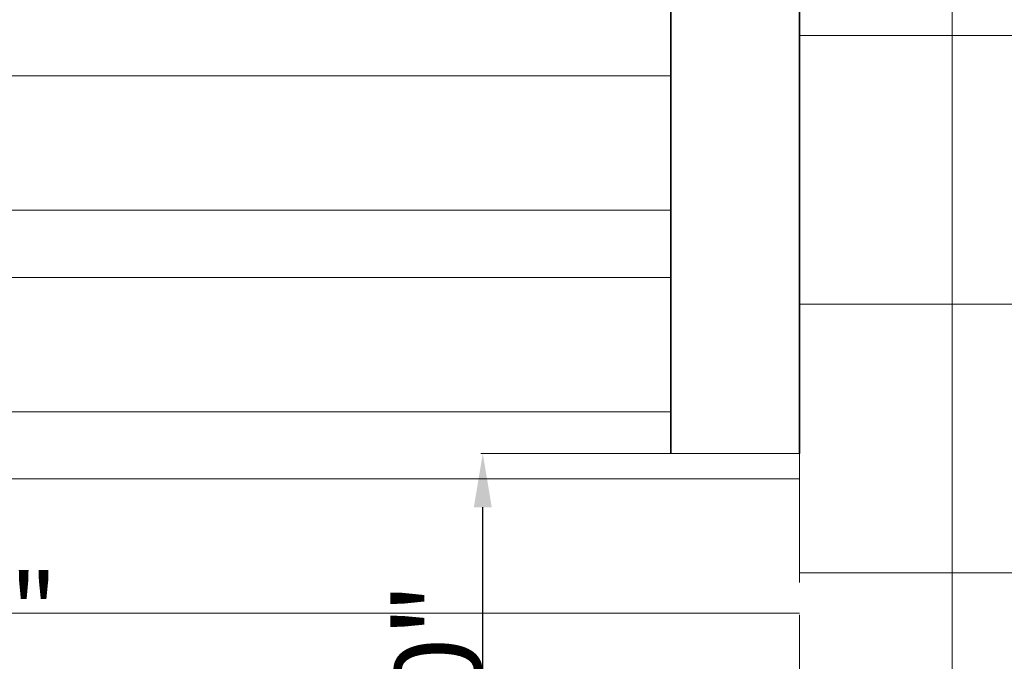
# Model space of a CAD drawing. Units: inches. Extents: x 351 to 1738, y -265 to 286.
# Tile 19 of 38: x 1176 to 1268, y -122 to -63. Entities that reach past the tile are written whole.
import ezdxf

# ---------------------------------------------------------------- set-up
doc = ezdxf.new("R2010")
doc.units = ezdxf.units.IN
doc.header["$MEASUREMENT"] = 0
doc.linetypes.add('ACAD_ISO02W100', pattern=[15, 12, -3])
for name, color, linetype, lineweight in [('A-ANNO-DIMS', 2, 'Continuous', 18), ('A-AREA-IDEN', 7, 'Continuous', 18), ('A-DOOR', 3, 'Continuous', 18), ('A-DOOR-OVHD', 3, 'ACAD_ISO02W100', 13), ('A-FLOR-PATT', 9, 'Continuous', 9), ('A-WALL', 7, 'Continuous', 35)]:
    doc.layers.add(name, color=color, linetype=linetype, lineweight=lineweight)
doc.styles.add('Annotative', font='arial.ttf')
doc.styles.get("Standard").update_dxf_attribs({"font": 'arial.ttf'})
doc.dimstyles.get("Standard").update_dxf_attribs({"dimtxt": 8, "dimasz": 5, "dimexe": 0.18, "dimexo": 0.0625, "dimgap": 0.09, "dimtad": 1, "dimtoh": 1, "dimzin": 0, "dimdsep": 46, "dimlunit": 4, "dimtxsty": 'Standard', "dimcen": 0, "dimclre": 256, "dimadec": 0, "dimazin": 0, "dimtfac": 1, "dimtofl": 0, "dimtmove": 0, "dimatfit": 3, "dimfxl": 1, "dimtolj": 1, "dimtzin": 0, "dimlwe": -1, "dimarcsym": 0})

# ---------------------------------------------------------------- blocks, each defined once
blk = doc.blocks.new('*D65')
at = {"layer": 'A-ANNO-DIMS', "transparency": 16777216}
for p, q in [((1248.45, -102.915), (1218.882, -102.915)), ((1248.45, -150.915), (1218.882, -150.915))]:
    blk.add_line(p, q, dxfattribs=at)
at = {"layer": 'A-ANNO-DIMS', "color": 0, "lineweight": -2, "transparency": 16777216}
blk.add_line((1219.062, -145.915), (1219.062, -107.915), dxfattribs=at)
at = {"layer": 'A-ANNO-DIMS', "color": 0, "transparency": 16777216}
for points in [[(1218.229, -107.915), (1219.896, -107.915), (1219.062, -102.915)], [(1218.229, -145.915), (1219.896, -145.915), (1219.062, -150.915)]]:
    blk.add_solid(points, dxfattribs=at)
at = {"layer": 'Defpoints', "color": 0, "transparency": 16777216}
for p in [(1219.062, -102.915), (1248.512, -102.915), (1248.512, -150.915)]:
    blk.add_point(p, dxfattribs=at)
at = {"layer": 'A-ANNO-DIMS', "color": 0, "transparency": 16777216, "insert": (1214.888, -126.915), "char_height": 8, "attachment_point": 5, "rotation": 90}
blk.add_mtext('\\A1;4\'-0"', dxfattribs=at)

msp = doc.modelspace()

# ---------------------------------------------------------------- hatches: boundary and pattern name
at = {"layer": 'A-FLOR-PATT', "transparency": 33554559}
h = msp.add_hatch(dxfattribs=at)
h.set_pattern_fill('ANSI37', color=256, scale=200, angle=135)
h.set_pattern_definition([(180, (1112.704, -164.037), (-2e-15, -25), []), (270, (1112.704, -164.037), (25, -5e-15), [])])
h.paths.add_polyline_path([(1380.064, 73.463), (1380.132, 148.463), (1338.064, 148.463), (1290.704, 148.463), (1290.704, 88.463), (1248.704, 88.463), (1248.704, -2.009), (1244.704, -2.009), (1244.704, 142.457), (1160.704, 142.457), (1160.704, 158.963), (1160.704, 170.137), (1160.704, 206.137), (1160.704, 228.963), (1112.704, 228.963), (1112.704, 209.963), (1112.704, 168.963), (1124.704, 168.963), (1124.704, 162.963), (1112.704, 162.963), (1112.704, 64.463), (1112.704, 60.463), (1112.704, 0.463), (1112.704, -48.026), (1146.804, -47.981), (1146.804, -35.691), (1207.804, -35.691), (1207.804, -47.902), (1236.542, -47.864), (1236.544, -50.009), (1248.5, -50.009), (1248.506, -102.915), (1248.512, -150.915), (1248.514, -164.037), (1248.549, -164.037), (1273.017, -164.037), (1273.017, -128.799), (1355.24, -128.799), (1355.24, -164.037), (1384.204, -164.037), (1384.204, -57.037), (1380.064, -57.037), (1380.064, -48.037), (1392.064, -48.037), (1392.064, -53.037), (1406.549, -53.037), (1406.549, -57.037), (1401.204, -57.037), (1401.204, -147.037), (1468.204, -147.037), (1468.204, -138.5), (1472.204, -138.5), (1472.204, -102.5), (1468.204, -102.5), (1468.204, -57.037), (1442.549, -57.037), (1442.549, -53.037), (1463.049, -53.037), (1463.049, -40.747), (1524.049, -40.747), (1524.049, -48.037), (1536.064, -48.037), (1536.064, -53.037), (1557.704, -53.037), (1557.704, 204.963), (1384.204, 204.963), (1384.204, 73.463), (1392.064, 73.463), (1392.064, 64.463), (1384.204, 64.463), (1384.204, -3.5), (1380.204, -3.537), (1380.204, 64.463), (1380.064, 64.463)])
h.paths.add_polyline_path([(1510.714, 86.458, -0.103984), (1511.661, 85.595, 0.470438), (1510.158, 87.614, 0.0961)], flags=16)
h.paths.add_polyline_path([(1510.443, 100.266, 0.009798), (1504.693, 100.48, 0.02879), (1504.6, 99.767, -0.165331), (1505.519, 96.135, -0.143601)], flags=16)
h.paths.add_polyline_path([(1487.201, 85.595, -0.103984), (1488.148, 86.458, 0.0961), (1488.704, 87.614, 0.470438)], flags=0)
h.paths.add_polyline_path([(1495.052, 100.43), (1494.178, 100.43, -0.026463), (1494.262, 99.774, -0.144219)], flags=16)
h.paths.add_polyline_path([(1444.485, 86.458, -0.103984), (1445.433, 85.595, 0.470438), (1443.93, 87.614, 0.0961)], flags=16)
h.paths.add_polyline_path([(1420.972, 85.595, -0.103984), (1421.92, 86.458, 0.0961), (1422.475, 87.614, 0.470438)], flags=16)
h.paths.add_polyline_path([(1428.632, 100.335, 0.001054), (1427.971, 100.309, -0.021524), (1428.033, 99.774, -0.114301)], flags=16)
h.paths.add_polyline_path([(1419.906, 143.708, 0.024979), (1420.222, 157.526), (1421.573, 159.101), (1421.573, 175.369), (1391.393, 175.369), (1391.393, 200.519), (1542.294, 200.519), (1542.294, 175.369), (1512.028, 175.369, 0.019865), (1511.521, 153.838, 0.025134), (1512.758, 118.323, 0.020553), (1512.942, 115.253), (1419.834, 115.253, -0.000414), (1419.843, 124.798), (1413.059, 124.798), (1413.059, 84.437, -0.061853), (1415.831, 80.45, -0.093077), (1420.972, 85.595, -0.267537), (1422.371, 84.732, 0.08511), (1424.052, 84.616, -0.885393), (1424.033, 84.851, -1.125815), (1424.073, 84.366, -0.087987), (1422.371, 84.732, -0.267537), (1422.326, 83.089, -0.370542), (1420.972, 85.595, 0.093077), (1415.831, 80.45, -0.087414), (1417.914, 73.937), (1418.941, 73.937, 0.02725), (1418.913, 76.906, -0.115703), (1421.051, 73.937), (1445.354, 73.937, -0.115703), (1447.492, 76.906, 0.02725), (1447.464, 73.937), (1448.491, 73.937, -0.087414), (1450.574, 80.45, 0.093077), (1445.433, 85.595, -0.370542), (1444.079, 83.089, -0.267537), (1444.034, 84.732, -0.087987), (1442.332, 84.366, -1.125815), (1442.372, 84.851, -2.032736), (1442.364, 84.368, 0.086378), (1444.034, 84.732, -0.267537), (1445.433, 85.595, -0.093077), (1450.574, 80.45, -0.257732), (1466.483, 90.927, -0.47867), (1468.832, 91.907, -0.47867), (1471.18, 90.927, -0.26264), (1483.053, 81.78, -0.071866), (1487.201, 85.595, -0.267537), (1488.6, 84.732, 0.08511), (1490.28, 84.616, -0.885393), (1490.262, 84.851, -1.125815), (1490.301, 84.366, -0.087987), (1488.6, 84.732, -0.267537), (1488.554, 83.089, -0.370542), (1487.201, 85.595, 0.071866), (1483.053, 81.78, -0.132065), (1484.143, 73.937), (1485.169, 73.937, 0.02725), (1485.142, 76.906, -0.115703), (1487.28, 73.937), (1511.582, 73.937, -0.115703), (1513.72, 76.906, 0.02725), (1513.693, 73.937), (1514.719, 73.937, -0.087414), (1516.802, 80.45, 0.093077), (1511.661, 85.595, -0.370542), (1510.308, 83.089, -0.267537), (1510.262, 84.732, -0.087987), (1508.561, 84.366, -1.125815), (1508.601, 84.851, -2.032736), (1508.592, 84.368, 0.086378), (1510.262, 84.732, -0.267537), (1511.661, 85.595, -0.093077), (1516.802, 80.45, -0.061853), (1519.575, 84.437), (1519.575, 73.937), (1413.059, 73.937), (1413.059, 124.798), (1419.843, 124.798, -0.000821)], flags=16)
h.paths.add_polyline_path([(1220.149, 54.133, -0.103984), (1220.869, 53.476, 0.470438), (1219.727, 55.011, 0.0961)], flags=16)
h.paths.add_polyline_path([(1219.944, 64.626, 0.009798), (1215.574, 64.789, 0.02879), (1215.503, 64.247, -0.165331), (1216.201, 61.487, -0.143601)], flags=16)
h.paths.add_polyline_path([(1209.779, 64.449, 0.097446), (1209.339, 64.751), (1208.247, 64.751, 0.12739), (1207.7, 64.326, 0.171586), (1206.95, 61.475, -0.158854), (1207.636, 59.45, 0.015898), (1207.795, 59.218, 0.061546), (1208.598, 59.616, 0.175416), (1208.638, 60.099, -0.284779), (1209.348, 62.472, 0.326216)], flags=16)
h.paths.add_polyline_path([(1169.818, 54.133, -0.103984), (1170.538, 53.476, 0.470438), (1169.396, 55.011, 0.0961)], flags=16)
h.paths.add_polyline_path([(1159.017, 62.472, 0.284764), (1158.307, 60.099, -0.175433), (1158.267, 59.616, 0.39293), (1159.448, 64.449, -0.32623)], flags=16)
h.paths.add_polyline_path([(1156.342, 58.239, -0.178321), (1154.011, 55.31, -0.174736), (1154.722, 55.233, -0.200802), (1156.27, 56.086, 0.12699), (1157.283, 58.991, -0.091205)], flags=16)
h.paths.add_polyline_path([(1156.624, 61.413, 0.157275), (1157.316, 64.247, 0.169622)], flags=16)
h.paths.add_polyline_path([(1152.67, 54.133, -0.0961), (1151.95, 53.476, 0.064076), (1154.465, 54.384, 0.199016)], flags=16)
h.paths.add_polyline_path([(1202.281, 53.476, -0.103984), (1203, 54.133, 0.0961), (1203.423, 55.011, 0.470438)], flags=0)
h.paths.add_polyline_path([(1151.139, 97.64, 0.024979), (1151.379, 108.141), (1152.406, 109.338), (1152.406, 121.701), (1129.47, 121.701), (1129.47, 140.814), (1244.149, 140.814), (1244.149, 121.701), (1221.148, 121.701, 0.019865), (1220.763, 105.338, 0.025134), (1221.703, 78.349, 0.020553), (1221.843, 76.016), (1151.078, 76.016, -0.128743), (1148.786, 65.037, 0.539352), (1150.327, 64.171, -0.027594), (1163.481, 64.751, 0.097695), (1163.04, 64.449, 0.326216), (1163.471, 62.472, -0.284777), (1164.181, 60.099, -0.194757), (1165.846, 61.443, -0.155402), (1165.172, 64.247, -0.166022), (1165.869, 61.475, -0.177014), (1167.852, 62.77, -0.448203), (1169.974, 60.807, -0.393499), (1167.679, 57.86, -0.895548), (1168.438, 54.524, -0.355767), (1166.218, 56.086, -0.066024), (1165.505, 57.539), (1165.251, 56.243, -0.371732), (1164.02, 59.758, -0.373614), (1163.04, 64.449, -0.097695), (1163.481, 64.751, 0.021354), (1153.294, 64.429, -0.134183), (1156.695, 61.368, 0.186873), (1154.636, 62.77, 0.448203), (1152.514, 60.807, 0.403726), (1154.905, 57.846, 0.711219), (1153.334, 55, 0.53154), (1151.95, 53.476, -0.267537), (1153.013, 52.821, 0.08511), (1154.29, 52.732, -0.885393), (1154.276, 52.911, -1.125815), (1154.306, 52.543, -0.087987), (1153.013, 52.821, -0.267537), (1152.978, 51.572, -0.370542), (1151.95, 53.476, 0.093077), (1148.043, 49.566, -0.087414), (1149.626, 44.617), (1150.406, 44.617, 0.02725), (1150.385, 46.873, -0.115703), (1152.01, 44.617), (1170.478, 44.617, -0.115703), (1172.103, 46.873, 0.02725), (1172.082, 44.617), (1172.862, 44.617, -0.087414), (1174.445, 49.566, 0.093077), (1170.538, 53.476, -0.370542), (1169.51, 51.572, -0.267537), (1169.475, 52.821, -0.087987), (1168.182, 52.543, -1.125815), (1168.212, 52.911, -2.032736), (1168.206, 52.544, 0.086378), (1169.475, 52.821, -0.267537), (1170.538, 53.476, -0.093077), (1174.445, 49.566, -0.257732), (1186.536, 57.528, -0.47867), (1188.321, 58.273, -0.47867), (1190.106, 57.528, -0.26264), (1199.128, 50.577, -0.071866), (1202.281, 53.476, -0.267537), (1203.344, 52.821, 0.08511), (1204.621, 52.732, -0.885393), (1204.607, 52.911, -1.125815), (1204.637, 52.543, -0.087987), (1203.344, 52.821, -0.267537), (1203.309, 51.572, -0.370542), (1202.281, 53.476, 0.071866), (1199.128, 50.577, -0.132065), (1199.957, 44.617), (1200.737, 44.617, 0.02725), (1200.716, 46.873, -0.115703), (1202.341, 44.617), (1220.809, 44.617, -0.115703), (1222.434, 46.873, 0.02725), (1222.413, 44.617), (1223.193, 44.617, -0.087414), (1224.776, 49.566, 0.093077), (1220.869, 53.476, -0.370542), (1219.841, 51.572, -0.267537), (1219.806, 52.821, -0.087987), (1218.513, 52.543, -1.125815), (1218.543, 52.911, -2.032736), (1218.537, 52.544, 0.086378), (1219.806, 52.821, -0.267537), (1220.869, 53.476, -0.093077), (1224.776, 49.566, -0.061853), (1226.883, 52.597), (1226.883, 44.617), (1145.936, 44.617), (1145.936, 83.269), (1151.091, 83.269, -0.000821)], flags=16)
h.paths.add_polyline_path([(1218.01, 57.86, -0.895548), (1218.769, 54.524, -0.355767), (1216.549, 56.086, -0.066024), (1215.836, 57.539), (1215.582, 56.243, -0.371732), (1214.351, 59.758, -0.373614), (1213.371, 64.449, 0.326216), (1213.802, 62.472, -0.284777), (1214.512, 60.099, -0.194757), (1216.177, 61.443, -0.179991), (1218.183, 62.77, -0.448203), (1220.305, 60.807, -0.393499)], flags=16)
h.paths.add_polyline_path([(1424.735, 91.363, -0.393499), (1421.715, 95.241, -0.448203), (1424.507, 97.824, -0.179991), (1427.147, 96.077, -0.194757), (1429.338, 94.309, -0.284777), (1430.272, 97.432, 0.326216), (1430.839, 100.034, -0.373614), (1429.55, 93.861, -0.371732), (1427.929, 89.235), (1427.596, 90.941, -0.066024), (1426.657, 89.029, -0.355767), (1423.736, 86.973, -0.895548)], flags=16)
h.paths.add_polyline_path([(1238.033, 131.257, -1), (1227.329, 131.257, -1)], flags=0)
h.paths.add_polyline_path([(1235.357, 131.257, -1), (1230.005, 131.257, -1)], flags=0)
h.paths.add_polyline_path([(1214.039, 54.243, 0.154382), (1214.38, 53.992, 0.358955), (1213.613, 54.016, 0.603948), (1214.379, 53.657, 0.371319), (1213.968, 52.872, 0.187994), (1214.312, 52.809, -0.592455), (1213.953, 52.967, -0.294279), (1214.083, 53.691, -1.300187), (1213.881, 54.134, -0.283762), (1214.469, 53.896, 1.15094)], flags=16)
h.paths.add_polyline_path([(1212.091, 56.286, -0.408434), (1211.337, 56.445, -0.036259), (1211.098, 56.848, -0.236098), (1211.59, 56.63, 0.035345), (1211.835, 56.543, -0.475241), (1212.091, 56.286, -0.475241), (1212.438, 56.182, 0.035345), (1212.631, 56.007, -0.236098), (1213.056, 55.676, -0.036259), (1212.588, 55.697, -0.408434)], flags=16)
h.paths.add_polyline_path([(1211.469, 50.297, 0.296043), (1210.47, 50.527, 0.310883), (1211.931, 50.148, 0.021255)], flags=16)
h.paths.add_polyline_path([(1213.739, 51.818, -0.036259), (1213.271, 51.838, -0.408434), (1212.774, 52.427, -0.094786), (1212.293, 50.703, 1.150474), (1212.911, 50.232, 0.166288), (1213.265, 50.68, -0.025254), (1212.603, 50.13, 1.087932), (1212.471, 49.407, 0.166288), (1213.02, 49.251, -0.016128), (1212.567, 49.563, -0.286859), (1212.217, 49.638, 0.022156), (1212.046, 50.055, -0.64613), (1212.185, 50.498, 0.088412), (1212.732, 52.077, -1.186037), (1213.121, 52.323, 0.035345), (1213.314, 52.148, -0.236098)], flags=16)
h.paths.add_polyline_path([(1212.094, 50.342, -0.048524), (1211.54, 49.605, -1.103834), (1211.397, 48.738, -0.785515), (1211.683, 48.254, -0.392043), (1210.948, 48.525, -0.392819), (1210.561, 47.995, -0.592455), (1210.201, 48.153, -0.294279), (1210.331, 48.877, -0.704172), (1210.316, 49.592, -0.679344), (1210.729, 50.112, 0.563676)], flags=16)
h.paths.add_polyline_path([(1211.274, 49.829, -0.139826), (1210.745, 49.859, -0.217879), (1210.948, 49.509, -0.498572)], flags=0)
h.paths.add_polyline_path([(1433.426, 81.49, -0.181571), (1434.245, 81.788, -0.008067), (1433.726, 82.205, 0.045578), (1432.755, 81.242, 0.179011)], flags=16)
h.paths.add_polyline_path([(1434.146, 81.009, -0.132442), (1433.645, 80.771, 0.259089), (1433.234, 80.471, -0.180211), (1433.392, 80.805, -0.16994), (1432.758, 81.109, 0.032652), (1433.273, 80.474, -0.493363), (1434.046, 80.146, -0.390497)], flags=16)
h.paths.add_polyline_path([(1434.83, 80.047, -0.947538), (1435.294, 79.576, -0.299128), (1434.625, 79.404, -0.270439), (1435.01, 78.591, -0.592455), (1434.537, 78.382, -0.392819), (1434.027, 79.08, -0.392043), (1433.06, 78.723, -0.352042), (1433.003, 79.197, -0.197216), (1433.75, 79.734, -0.71364), (1434.447, 79.939, -0.21479), (1434.819, 80.475, 0.408833), (1435.075, 80.803, -0.226152)], flags=16)
h.paths.add_polyline_path([(1432.67, 81.217, -0.454218), (1431.897, 79.923, -0.414411), (1431.301, 80.035, 0.016129), (1431.897, 80.445, 0.27957), (1432.073, 80.871, -0.289504), (1431.103, 81.321, -0.414411), (1430.978, 81.915, 0.01613), (1431.586, 81.521, 0.341293), (1432.125, 81.583, -0.813186)], flags=16)
h.paths.add_polyline_path([(1429.893, 86.381, -0.947538), (1430.358, 85.91, -0.173106), (1429.984, 85.712, -0.038817), (1431.625, 84.214, -0.0879), (1432.097, 88.549, -0.049768), (1431.254, 88.49, -0.236098), (1431.814, 88.925, 0.035345), (1432.067, 89.155, -0.475241), (1432.524, 89.291, -0.475241), (1432.86, 89.63, 0.035345), (1433.182, 89.744, -0.236098), (1433.83, 90.032, -0.036259), (1433.516, 89.502, -0.408434), (1432.524, 89.291, -0.312424), (1432.106, 88.58, 0.088559), (1431.625, 84.214, -0.408434), (1430.971, 83.439, -0.036259), (1430.355, 83.412, -0.236098), (1430.914, 83.847, 0.035345), (1431.168, 84.078, -0.475241), (1431.625, 84.214, 0.038817), (1429.984, 85.712, -0.321732), (1429.333, 86.048, -0.32743), (1429.883, 86.809, 0.408833), (1430.138, 87.138, -0.226152)], flags=16)
h.paths.add_polyline_path([(1211.206, 58.616, -0.999784), (1211.336, 59.323, -0.614994)], flags=16)
h.paths.add_polyline_path([(1210.288, 49.429, 0.154382), (1210.629, 49.178, 0.358955), (1209.861, 49.202, 0.603948), (1210.627, 48.843, -0.534825), (1210.806, 49.295, 0.748346)], flags=16)
h.paths.add_polyline_path([(1209.589, 51.828, -0.008791), (1209.775, 51.753, 0.112231), (1209.466, 52.019, 1.418851), (1209.014, 51.708, -0.458726), (1208.651, 51.073, -0.592455), (1208.291, 51.232, -0.294279), (1208.421, 51.955, -1.300187), (1208.219, 52.398, -0.226005), (1208.719, 52.257, -0.475519), (1209.158, 52.369, -1.455499), (1209.603, 52.664, 0.421305), (1209.191, 52.262, -0.591212), (1208.979, 51.796, 0.497399), (1209.773, 51.333, 0.649312)], flags=16)
h.paths.add_polyline_path([(1208.029, 52.041, 0.544667), (1208.832, 52.045, 0.220132)], flags=0)
h.paths.add_polyline_path([(1210.438, 51.425, -0.2042), (1210.277, 52.018, 0.270826), (1209.915, 52.897, 0.324115)], flags=0)
h.paths.add_polyline_path([(1209.668, 52.407, -0.60139), (1208.99, 52.221, -0.394916), (1208.248, 52.83, -0.836792), (1208.651, 53.017, -0.338488), (1209.039, 52.571, 0.194138), (1209.191, 52.262, 0.413995), (1209.712, 52.475, 0.51771), (1210.503, 51.416, 0.401922), (1209.493, 50.93, 0.206396), (1209.516, 50.165, -0.319463), (1210.417, 51.418, -0.466635)], flags=16)
h.paths.add_polyline_path([(1206.601, 56.086, -0.355767), (1204.381, 54.524, -0.921198), (1205.236, 57.846, 0.206569), (1207.614, 58.991, -0.12699)], flags=16)
h.paths.add_polyline_path([(1435.487, 82.816, 0.527765), (1436.615, 83.361, 0.50854), (1437.05, 82.433, 0.592455), (1437.524, 82.641, 0.331245), (1436.963, 83.548, 0.387863), (1437.808, 83.626, 0.592954), (1437.618, 84.176, 0.226016), (1436.961, 83.99, 0.318205), (1437.588, 84.854, 0.689374), (1437.05, 84.991, 0.335765), (1436.539, 84.41, -0.156993), (1436.404, 84.065, -0.434611), (1436.961, 83.99, -0.21479), (1437.333, 84.526, 0.408833), (1437.588, 84.854, -0.226152), (1437.343, 84.097, -0.947538), (1437.808, 83.626, -0.299128), (1437.139, 83.455, -0.270439), (1437.524, 82.641, -0.592455), (1437.05, 82.433, -0.392819), (1436.541, 83.13, -0.43966), (1435.475, 82.794, -0.174614), (1435.942, 82.244, -0.206396), (1435.912, 81.237, -0.270826), (1435.125, 82.208, 0.207976), (1434.686, 82.904, -0.196495)], flags=16)
h.paths.add_polyline_path([(1435.386, 84.832, 0.270811), (1434.91, 83.676, -0.204217), (1434.699, 82.895, 0.324115)], flags=0)
h.paths.add_polyline_path([(1435.68, 84.18, -0.217656), (1435.554, 83.304, -0.176705), (1436.236, 83.778, -0.373036)], flags=0)
h.paths.add_polyline_path([(1435.566, 100.034, 0.326216), (1436.133, 97.432, -0.284777), (1437.067, 94.309, -0.194757), (1439.258, 96.077, -0.155402), (1438.371, 99.767, -0.166022), (1439.289, 96.12, -0.177014), (1441.897, 97.824, -0.448203), (1444.69, 95.241, -0.393499), (1441.67, 91.363, -0.895548), (1442.669, 86.973, -0.355767), (1439.748, 89.029, -0.066024), (1438.809, 90.941), (1438.476, 89.235, -0.371732), (1436.855, 93.861, -0.373614)], flags=16)
h.paths.add_polyline_path([(1191.252, 49.507, -0.274022), (1190.658, 48.409, 0.267537), (1191.311, 47.344, 0.370542)], flags=0)
h.paths.add_polyline_path([(1190.301, 49.717, 0.199016), (1188.619, 49.04, 0.064076), (1191.252, 49.507, -0.0961)], flags=0)
h.paths.add_polyline_path([(1189.518, 47.857, 1.125815), (1189.676, 47.523, 2.044605)], flags=0)
h.paths.add_polyline_path([(1464.974, 80.372, 0.274022), (1465.756, 78.927, -0.083013)], flags=0)
h.paths.add_polyline_path([(1464.974, 80.372, 0.370542), (1464.897, 77.525, 0.576324)], flags=0)
h.paths.add_polyline_path([(1464.974, 80.372, -0.470438), (1467.284, 81.372, -0.0961), (1466.226, 80.648, -0.199016), (1468.439, 79.757, -0.064076)], flags=0)
h.paths.add_polyline_path([(1189.511, 56.43, -0.259467), (1188.321, 56.391, -0.259467), (1187.13, 56.43, 0.08511), (1188.193, 55.716, -0.885393), (1188.27, 55.878, -1.196013), (1188.355, 55.442, 0.101459)], flags=0)
h.paths.add_polyline_path([(1188.321, 57.596, 0.078072), (1187.678, 57.24, 0.01555), (1188.321, 57.136, 0.01555), (1188.964, 57.24, 0.078072)], flags=0)
h.paths.add_polyline_path([(1190.164, 55.365, -0.576324), (1190.106, 57.528, -0.198294), (1188.321, 58.319, -0.198294), (1186.536, 57.528, -0.576324), (1186.477, 55.365, -0.370542), (1186.536, 57.528, 0.198294), (1188.321, 58.319, 0.198294), (1190.106, 57.528, -0.370542)], flags=0)
h.paths.add_polyline_path([(1188.372, 55.878, 1.125814), (1188.529, 55.544, 2.044605)], flags=0)
h.paths.add_polyline_path([(1186.341, 49.717, -0.0961), (1185.389, 49.507, 0.064076), (1188.022, 49.04, 0.199016)], flags=0)
h.paths.add_polyline_path([(1185.389, 49.507, -0.267537), (1185.984, 48.409, 0.08511), (1187.046, 47.695, -0.885393), (1187.123, 47.857, -1.125815), (1186.966, 47.523, -0.087987), (1185.984, 48.409, -0.267537), (1185.331, 47.344, -0.370542)], flags=0)
h.paths.add_polyline_path([(1399.441, 187.944, -1), (1413.525, 187.944, -1)], flags=0)
h.paths.add_polyline_path([(1402.962, 187.944, -1), (1410.004, 187.944, -1)], flags=0)
h.paths.add_polyline_path([(1357.663, -72.245), (1377.272, -72.245), (1377.272, -91.854), (1357.663, -91.854)], flags=16)
h.paths.add_polyline_path([(1467.256, 78.201, -1.125815), (1467.049, 77.761, -2.044605)], flags=0)
h.paths.add_polyline_path([(1468.822, 88.714, 0.941125), (1469.106, 88.316, 1.137152), (1468.765, 88.755, 0.890986), (1468.99, 88.245, 0.094828), (1470.398, 89.481, -0.267537), (1471.18, 90.927, -0.028123), (1469.678, 90.547, -0.028774), (1469.948, 90.311, -0.020327), (1468.832, 90.41, -0.020327), (1467.716, 90.311, -0.028774), (1467.986, 90.547, -0.028123), (1466.483, 90.927, -0.267537), (1467.265, 89.481, 0.08511), (1468.663, 88.542, -1.202316)], flags=0)
h.paths.add_polyline_path([(1178.25, 124.523, -0.119929), (1165.65, 124.145, -0.107349), (1159.133, 124.446, -0.102891), (1159.132, 130.465, -0.074897), (1158.993, 137.956, 0.002027), (1167.844, 137.479, -0.07553), (1180.337, 137.666, -0.075861), (1186.502, 137.688, -0.14099), (1186.272, 130.046, -0.095481), (1186.729, 124.748, -0.10603)], flags=0)
h.paths.add_polyline_path([(1469.225, 79.757, -0.199016), (1471.437, 80.648, -0.0961), (1470.379, 81.372, -0.470438), (1472.689, 80.372, -0.370542), (1472.766, 77.525, -0.267537), (1471.907, 78.927, -0.087986), (1470.615, 77.761, -1.125849), (1470.408, 78.201, -2.032736), (1470.642, 77.778, 0.086378), (1471.907, 78.927, -0.267537), (1472.689, 80.372, -0.064076)], flags=0)
h.paths.add_polyline_path([(1430.423, 186.902, -0.074897), (1430.24, 196.758, 0.002027), (1441.887, 196.131, -0.07553), (1458.326, 196.377, -0.075861), (1466.438, 196.406, -0.14099), (1466.136, 186.35, -0.095481), (1466.737, 179.378, -0.10603), (1455.58, 179.082, -0.119929), (1439, 178.585, -0.107349), (1430.425, 178.981, -0.102891)], flags=0)
h.paths.add_polyline_path([(1162.258, 49.939, 0.335765), (1161.87, 49.497, -0.156994), (1161.767, 49.235, -0.434611), (1162.19, 49.178, -0.21479), (1162.473, 49.585, 1.529195)], flags=16)
h.paths.add_polyline_path([(1161.683, 49.021, 0.581518), (1161.268, 49.583, 0.592761)], flags=16)
h.paths.add_polyline_path([(1162.602, 48.058, 0.371319), (1162.192, 48.843, 0.434533), (1162.88, 48.962, 0.185081), (1162.197, 48.926, 1.121837)], flags=16)
h.paths.add_polyline_path([(1161.443, 48.941, -1.307104), (1161.495, 48.571, -0.217752), (1161.136, 48.254, 0.697303), (1161.871, 49.048, 0.121514)], flags=16)
h.paths.add_polyline_path([(1162.531, 49.429, -0.207084), (1162.05, 49.146, -0.99203)], flags=16)
h.paths.add_polyline_path([(1161.304, 49.578, -0.719667), (1161.513, 50.079, -0.130428), (1160.836, 50.168, 0.039593)], flags=0)
h.paths.add_polyline_path([(1162.036, 50.584, -0.008067), (1161.642, 50.9, 0.029367), (1161.35, 50.297, -0.205788)], flags=16)
h.paths.add_polyline_path([(1162.882, 51.392, -0.124733), (1162.763, 51.828, -0.101191), (1162.399, 51.438, -0.153425)], flags=0)
h.paths.add_polyline_path([(1164.235, 51.85, -0.309107), (1164.513, 51.136, -0.627125), (1163.781, 51.603, -0.685909), (1162.777, 51.219, -0.233285), (1163.303, 50.165, -0.270826), (1162.705, 50.903, 0.2042), (1162.381, 51.425, 0.204182), (1162.542, 52.018, -0.270841), (1162.903, 52.897, -0.127261), (1163.219, 52.529, -1.168681), (1163.781, 52.587, -0.329112), (1164.168, 53.017, -0.836792), (1164.571, 52.83, -0.193341), (1164.391, 52.338, -0.947538), (1164.744, 51.981, -0.299128)], flags=16)
h.paths.add_polyline_path([(1163.598, 51.937, -1.262956), (1163.236, 51.831, 0.012575), (1162.971, 51.721, 0.230657), (1163.151, 52.407, -0.164898), (1163.178, 52.661, -0.44932), (1163.628, 52.262, -0.721477), (1164.154, 52.088, -0.849998)], flags=0)
h.paths.add_polyline_path([(1161.613, 58.616, -0.980413), (1161.525, 59.049, -2.908935)], flags=16)
h.paths.add_polyline_path([(1160.252, 49.166, -0.414411), (1159.799, 49.251, 0.016129), (1160.252, 49.563, 0.27957), (1160.386, 49.887, -0.289504), (1159.649, 50.229, -0.414411), (1159.554, 50.68, 0.01613), (1160.015, 50.381, 0.617885), (1160.526, 50.703, -0.094786), (1160.045, 52.427, -0.140444), (1159.682, 52.042, -0.057856), (1159.3, 51.872, 0.544843), (1160.046, 52.419, -0.088122), (1160.404, 55.721, -0.049768), (1159.763, 55.676, -0.236098), (1160.188, 56.007, 0.035345), (1160.381, 56.182, -0.475241), (1160.728, 56.286, -0.475241), (1160.984, 56.543, 0.035345), (1161.229, 56.63, -0.236098), (1161.721, 56.848, -0.036259), (1161.482, 56.445, -0.408434), (1160.728, 56.286, -0.312424), (1160.411, 55.745, 0.088559), (1160.045, 52.427, 0.107081), (1160.634, 50.498, -0.494798), (1160.839, 50.149, -0.454218)], flags=16)
h.paths.add_polyline_path([(1160.666, 49.808, -2.076528), (1160.828, 50.172, 0.019586)], flags=0)
h.paths.add_polyline_path([(1158.439, 53.992, 0.154382), (1158.78, 54.243, 0.748346), (1158.262, 54.109, -0.338225), (1158.492, 53.839, -0.170816), (1159.124, 53.779, 0.495729), (1158.938, 54.134, 0.226016)], flags=16)
h.paths.add_polyline_path([(1160.045, 52.427, 0.038817), (1158.798, 53.565, -0.119818), (1158.574, 53.586, -0.309107), (1158.851, 52.872, -0.187994), (1158.506, 52.809, 0.592455), (1158.866, 52.967, 0.331245), (1158.44, 53.657, 0.201245), (1158.798, 53.565, -0.034023), (1159.901, 52.578, -0.044253), (1159.698, 52.323, -0.475241)], flags=16)
h.paths.add_polyline_path([(1336.926, -95.392), (1336.926, -117.945), (1291.82, -117.945), (1291.82, -95.392)], flags=16)
h.paths.add_polyline_path([(1357.535, -97.244), (1357.726, -96.697, 0.034844)], flags=16)
h.paths.add_polyline_path([(1376.693, -96.478), (1377.301, -96.5, 0.031497), (1375.907, -96.424), (1357.726, -96.424)], flags=16)
h.paths.add_polyline_path([(1379.403, -119.667, 0.026706), (1380.043, -119.439, -0.015299)], flags=16)
h.paths.add_polyline_path([(1357.726, -120.202), (1357.821, -120.202), (1357.821, -120.201)], flags=16)
h.paths.add_polyline_path([(1354.171, -104.592), (1354.469, -98.672, 0.011138)], flags=16)
h.paths.add_polyline_path([(1355.058, -119.136), (1354.578, -118.539, 0.143164)], flags=16)
h.paths.add_polyline_path([(1378.851, -96.821), (1378.85, -96.82), (1378.85, -96.82, -0.04968), (1380.055, -97.191), (1378.85, -96.82, 0.150054), (1375.135, -97.188), (1375.136, -119.44, -0.00997), (1374.747, -116.649), (1357.726, -116.649, 0.169385), (1357.535, -119.382), (1357.535, -119.382), (1357.535, -119.382, 0.034818), (1357.726, -119.928), (1357.726, -119.928), (1357.726, -119.929, -0.034877), (1357.535, -119.382), (1355.507, -119.382), (1355.317, -119.278), (1357.535, -119.382, -0.169394), (1357.726, -116.649, -0.039151), (1374.686, -116.113, -0.002015), (1374.625, -115.546, 0.115322), (1369.915, -115.474, 0.060921), (1369.922, -101.154, 0.115146), (1374.625, -101.079, -0.002016), (1374.686, -100.513, -0.039151), (1357.726, -99.977), (1374.747, -99.977, -0.009963), (1375.135, -97.188), (1375.135, -97.188, -0.150108)], flags=16)
h.paths.add_polyline_path([(1490.963, 91.363, -0.393499), (1487.944, 95.241, -0.448203), (1490.736, 97.824, -0.179991), (1493.376, 96.077, -0.194757), (1495.567, 94.309, -0.284777), (1496.501, 97.432, 0.326216), (1497.068, 100.034, -0.373614), (1495.778, 93.861, -0.371732), (1494.158, 89.235), (1493.824, 90.941, -0.066024), (1492.886, 89.029, -0.355767), (1489.964, 86.973, -0.895548)], flags=16)
h.paths.add_polyline_path([(1354.86, -97.658), (1355.316, -97.348, 0.101911)], flags=16)
h.paths.add_polyline_path([(1497.063, 83.327, 0.176724), (1496.37, 83.785, -0.405139), (1496.016, 83.384, 0.497399), (1497.06, 82.774, 0.649312), (1496.818, 83.426, -0.008791)], flags=16)
h.paths.add_polyline_path([(1496.339, 83.783, 0.592761), (1496.886, 84.522, 0.581518)], flags=16)
h.paths.add_polyline_path([(1495.11, 82.641, 0.592455), (1495.583, 82.433, 0.676915), (1495.805, 83.59, 0.375669)], flags=16)
h.paths.add_polyline_path([(1495.015, 84.176, -0.145057), (1495.301, 84.526, -0.408833), (1495.045, 84.854, 0.220629), (1495.381, 84.152, -0.199594), (1495.851, 83.764, -0.524017), (1494.826, 83.626, -0.592998)], flags=16)
h.paths.add_polyline_path([(1501.655, 81.915, -0.016129), (1501.048, 81.521, -0.392719), (1500.462, 81.37, -0.21067), (1500.607, 81.142, 0.306699)], flags=16)
h.paths.add_polyline_path([(1500.11, 89.291, -0.408434), (1499.118, 89.502, -0.036259), (1498.803, 90.032, -0.236098), (1499.451, 89.744, 0.035345), (1499.774, 89.63, -0.475241), (1500.11, 89.291, -0.475241), (1500.567, 89.155, 0.035345), (1500.82, 88.925, -0.236098), (1501.379, 88.49, -0.036259), (1500.763, 88.516, -0.408434)], flags=16)
h.paths.add_polyline_path([(1498.908, 82.205, -0.051322), (1500.013, 81.134, -0.587931), (1500.234, 81.676, 0.107081), (1501.009, 84.214, -0.03529)], flags=16)
h.paths.add_polyline_path([(1496.93, 83.875, -0.206396), (1497.247, 84.832, -0.270826), (1497.724, 83.676, 0.207976), (1497.944, 82.884, -0.381455)], flags=16)
h.paths.add_polyline_path([(1496.721, 81.237, 0.270812), (1497.509, 82.208, -0.204216), (1497.935, 82.895, 0.324115)], flags=16)
h.paths.add_polyline_path([(1497.529, 80.125, -0.145057), (1497.814, 80.475, -0.703182), (1498.282, 81.178, -0.122925), (1497.977, 81.714, -0.270837), (1499.207, 81.49, 0.207964), (1499.993, 81.248, -0.265145), (1499.278, 80.472, 0.381901), (1498.808, 79.947, -0.305905), (1498.848, 79.519, 0.499482), (1498.574, 79.217, -0.458726), (1498.097, 78.382, -0.592455), (1497.624, 78.591, -0.270439), (1498.009, 79.404, -0.299116), (1497.34, 79.576, -0.593016)], flags=16)
h.paths.add_polyline_path([(1500.736, 79.923, 0.414411), (1501.333, 80.035, -0.321648), (1500.192, 80.765, 0.019886), (1499.976, 81.251, 0.465331)], flags=16)
h.paths.add_polyline_path([(1501.009, 84.214, -0.038817), (1502.649, 85.712, -0.173095), (1502.276, 85.91, -0.593016), (1502.465, 86.46, -0.145057), (1502.751, 86.809, -0.408833), (1502.495, 87.138, 0.220629), (1502.831, 86.436, -0.199594), (1503.301, 86.048, -0.321732), (1502.649, 85.712, 0.038817), (1501.009, 84.214, 0.122449), (1501.412, 83.755, 0.475491), (1501.335, 84.226, 0.055822), (1501.719, 83.847, -0.236098), (1502.278, 83.412, -0.036259), (1501.663, 83.439, -0.408434)], flags=16)
h.paths.add_polyline_path([(1501.794, 100.034, 0.326216), (1502.362, 97.432, -0.284777), (1503.295, 94.309, -0.194757), (1505.486, 96.077, -0.179991), (1508.126, 97.824, -0.448203), (1510.918, 95.241, -0.393499), (1507.899, 91.363, -0.895548), (1508.898, 86.973, -0.355767), (1505.976, 89.029, -0.066024), (1505.038, 90.941), (1504.704, 89.235, -0.371732), (1503.084, 93.861, -0.373614)], flags=16)
h.paths.add_polyline_path([(1146.29, 131.257, -1), (1135.587, 131.257, -1)], flags=0)
h.paths.add_polyline_path([(1143.614, 131.257, -1), (1138.262, 131.257, -1)], flags=0)
h.paths.add_polyline_path([(1524.064, 73.463), (1536.064, 73.463), (1536.064, 64.463), (1524.064, 64.463)], flags=16)
h.paths.add_polyline_path([(1520.162, 187.944, -1), (1534.246, 187.944, -1)], flags=0)
h.paths.add_polyline_path([(1530.725, 187.944), (1527.204, 187.944), (1527.204, 184.423, 0.414214)], flags=0)
h.paths.add_polyline_path([(1278.415, -91.154), (1331.067, -91.154), (1331.067, -80.583), (1278.415, -80.583)], flags=24)
h.paths.add_polyline_path([(1266.655, -79.354), (1354.738, -79.354), (1354.738, -67.817), (1266.655, -67.817)], flags=24)
h.paths.add_polyline_path([(1115.482, 206.184), (1155.098, 206.184), (1155.098, 217.714), (1115.482, 217.714)], flags=24)
h.paths.add_polyline_path([(1161.771, 8.501), (1222.466, 8.501), (1222.466, 19.079), (1161.771, 19.079)], flags=24)
h.paths.add_polyline_path([(1164.656, 18.795), (1210.615, 18.795), (1210.615, 30.324), (1164.656, 30.324)], flags=24)
h.paths.add_polyline_path([(1368.147, -32.882), (1379.362, -32.882), (1379.362, -21.733), (1368.147, -21.733)], flags=24)
h.paths.add_polyline_path([(1244.842, -31.012), (1256.057, -31.012), (1256.057, -19.863), (1244.842, -19.863)], flags=24)
h.paths.add_polyline_path([(1114.589, 195.739), (1156.517, 195.739), (1156.517, 206.31), (1114.589, 206.31)], flags=24)
h.paths.add_polyline_path([(1436.398, 37.632), (1505.131, 37.632), (1505.131, 48.203), (1436.398, 48.203)], flags=24)
h.paths.add_polyline_path([(1435.991, 47.919), (1507.906, 47.919), (1507.906, 59.456), (1435.991, 59.456)], flags=24)
h.paths.add_polyline_path([(1415.107, -124.896), (1457.038, -124.896), (1457.038, -114.318), (1415.107, -114.318)], flags=24)
h.paths.add_polyline_path([(1417.992, -114.602), (1457.609, -114.602), (1457.609, -103.073), (1417.992, -103.073)], flags=24)
h = msp.add_hatch(dxfattribs=at)
h.set_pattern_fill('ANSI32', color=256, scale=50, angle=135)
h.set_pattern_definition([(180, (1038.704, -199.037), (-2e-15, -18.75), []), (180, (1032.454, -192.787), (-2e-15, -18.75), [])])
h.paths.add_polyline_path([(1248.506, -102.915), (1236.559, -102.916), (1236.553, -56.864), (1112.704, -57.026), (1112.704, -57.037), (1103.704, -57.037), (1103.704, -45.037), (1103.704, 98.963), (1076.434, 98.963), (1076.549, -81.037), (1071.549, -81.037), (1043.704, -81.037), (1038.704, -81.037), (1038.704, -161.037), (1043.704, -161.037), (1043.704, -173.037), (1038.704, -173.037), (1038.704, -199.037), (1562.704, -199.037), (1562.704, -173.037), (1236.549, -173.037), (1236.549, -164.037), (1236.693, -164.037), (1236.676, -150.916), (1248.512, -150.915)])
h.paths.add_polyline_path([(1236.133, -134.078), (1247.348, -134.078), (1247.348, -122.929), (1236.133, -122.929)], flags=24)
h.paths.add_polyline_path([(1308.144, -185.548), (1321.66, -185.548), (1321.66, -174.4), (1308.144, -174.4)], flags=24)
h.paths.add_polyline_path([(1121.632, -122.88), (1179.647, -122.88), (1179.647, -112.309), (1121.632, -112.309)], flags=24)
h.paths.add_polyline_path([(1124.515, -112.593), (1177.986, -112.593), (1177.986, -101.056), (1124.515, -101.056)], flags=24)
h.paths.add_polyline_path([(1091.374, 23.58), (1104.89, 23.58), (1104.89, 34.728), (1091.374, 34.728)], flags=24)

# ---------------------------------------------------------------- linework, layer by layer
at = {"layer": 'A-DOOR'}
msp.add_line((1236.676, -102.916), (1248.512, -102.915), dxfattribs=at)
at = {"layer": 'A-DOOR-OVHD'}
msp.add_line((1248.506, -102.915), (1248.512, -150.915), dxfattribs=at)
at = {"layer": 'A-WALL'}
for p, q in [((1248.5, -50.009), (1248.506, -102.915)), ((1236.553, -56.864), (1236.559, -102.916))]:
    msp.add_line(p, q, dxfattribs=at)

# ---------------------------------------------------------------- texts
at = {"layer": 'A-AREA-IDEN', "style": 'Annotative'}
msp.add_text('16\'10"X12\'6"', height=6.90137, dxfattribs=at).set_placement((1123.394, -121))

# ---------------------------------------------------------------- dimensions: what is measured, and where the dimension line sits
at = {"layer": 'A-ANNO-DIMS'}
dim = msp.add_linear_dim(base=(1219.062, -102.915), p1=(1248.512, -150.915), p2=(1248.512, -102.915), angle=90, dimstyle='Standard', override={"dimdec": 1, "dimlfac": 1, "dimrnd": 0, "dimzin": 1, "dimdsep": 46, "dimlunit": 4, "dimfrac": 2}, dxfattribs=at)
dim.commit()
dim.dimension.update_dxf_attribs({"geometry": '*D65', "text_midpoint": (1214.888, -126.915)})

doc.saveas('drawing.dxf')
